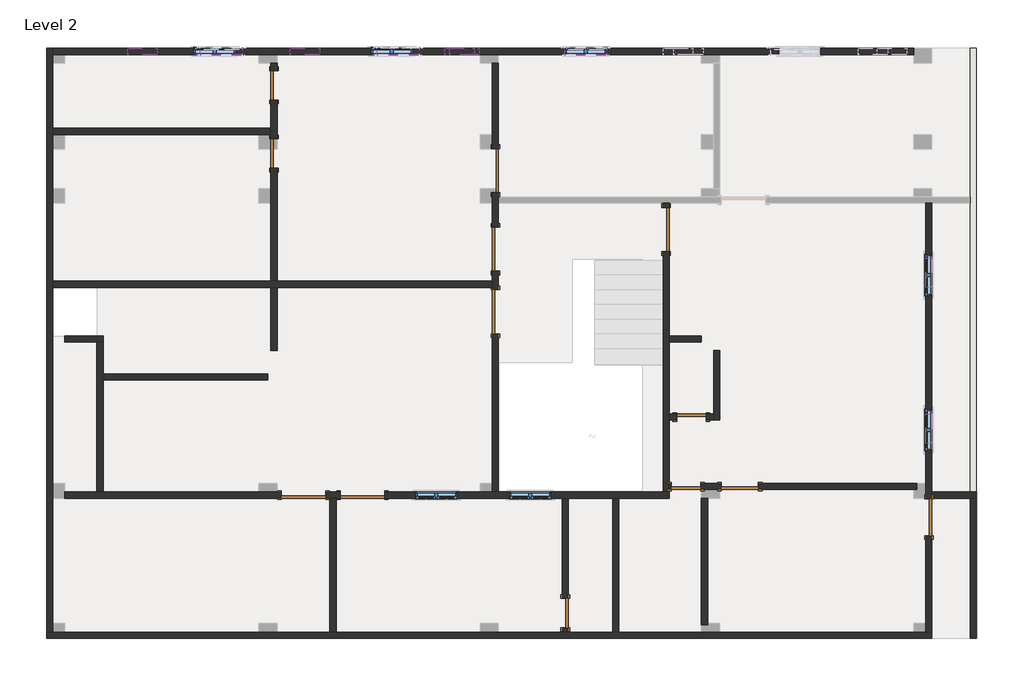
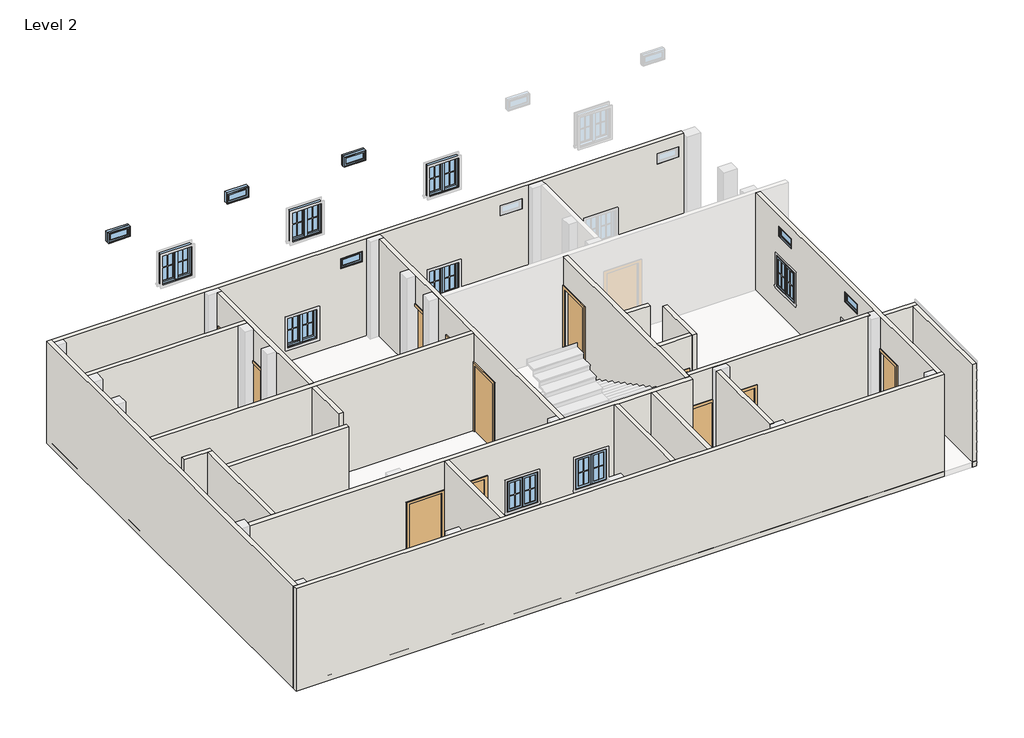
# One storey, part 1 of 2: 24 walls, 16 windows, 13 doors.
"""IFC4 building model written with IfcOpenShell, lengths in millimetres."""

from ifc_helpers import new_model, si_unit, frame, origin, place, context, project, spatial, polyline, outline, extrude, faceted_brep, transform, mapped, element, save
from components import single_flush_2_ccebbf4d, single_flush_2_025d1c86, door_e00f436c, door_1fe7f57d, door_a3eb833a, door_a1797ceb, window_4c2727af, window_0d9958e7

model = new_model("IFC4")

# Units and contexts
model_context = context("Model", 3, world=origin())
ifc_project = project(units=[si_unit("LENGTHUNIT", "METRE", prefix="MILLI")], contexts=[model_context])

# Site, building, storey
site = spatial("IfcSite", under=ifc_project)
building = spatial("IfcBuilding", under=site)
storey = spatial("IfcBuildingStorey", under=building, Name="Level 2", Elevation=3048.0)

# Doors
placement = place(None, origin())
single_flush_2_shape = single_flush_2_ccebbf4d(model_context)
element("IfcDoor", 1, ObjectType="Single-Flush : 2'", at=placement, inside=storey, context=model_context, shape_type="MappedRepresentation", body=[
    mapped(single_flush_2_shape, transform((758.239606, -5823.8831508, 3048.0), x_axis=(1.0, 0.0, 0.0), y_axis=(0.0, 1.0, 0.0), z_axis=(0.0, 0.0, 1.0))),
])
element("IfcDoor", 2, ObjectType="Single-Flush : 2'", at=placement, inside=storey, context=model_context, shape_type="MappedRepresentation", body=[
    mapped(single_flush_2_shape, transform((874.8985263, -4388.7831508, 3048.0), x_axis=(-1.0, 0.0, 0.0), y_axis=(0.0, -1.0, 0.0), z_axis=(0.0, 0.0, 1.0))),
])
single_flush_2_2_shape = single_flush_2_025d1c86(model_context)
element("IfcDoor", 3, ObjectType="Single-Flush : 2'", at=placement, inside=storey, context=model_context, shape_type="MappedRepresentation", body=[
    mapped(single_flush_2_2_shape, transform((-1732.230394, -8440.0831508, 3048.0), x_axis=(0.0, -1.0, 0.0), y_axis=(1.0, 0.0, 0.0), z_axis=(0.0, 0.0, 1.0))),
])
element("IfcDoor", 4, ObjectType="Single-Flush : 2'", at=placement, inside=storey, context=model_context, shape_type="MappedRepresentation", body=[
    mapped(single_flush_2_2_shape, transform((-7746.0425534, 2469.2168492, 3048.0), x_axis=(0.0, 1.0, 0.0), y_axis=(-1.0, 0.0, 0.0), z_axis=(0.0, 0.0, 1.0))),
])
element("IfcDoor", 5, ObjectType="Single-Flush : 2'", at=placement, inside=storey, context=model_context, shape_type="MappedRepresentation", body=[
    mapped(single_flush_2_2_shape, transform((-7746.0425534, 1059.5168492, 3048.0), x_axis=(0.0, 1.0, 0.0), y_axis=(-1.0, 0.0, 0.0), z_axis=(0.0, 0.0, 1.0))),
])
door_shape = door_e00f436c(model_context)
element("IfcDoor", 6, ObjectType="Single-Flush : 30\" x 80\"", at=placement, inside=storey, context=model_context, shape_type="MappedRepresentation", body=[
    mapped(door_shape, transform((5779.4574466, -6458.8831508, 3048.0), x_axis=(0.0, 1.0, 0.0), y_axis=(-1.0, 0.0, 0.0), z_axis=(0.0, 0.0, 1.0))),
])
door_2_shape = door_1fe7f57d(model_context)
element("IfcDoor", 7, ObjectType="Single-Flush : 30\" x 80\"", at=placement, inside=storey, context=model_context, shape_type="MappedRepresentation", body=[
    mapped(door_2_shape, transform((1875.839606, -5823.8831508, 3048.0), x_axis=(-1.0, 0.0, 0.0), y_axis=(0.0, -1.0, 0.0), z_axis=(0.0, 0.0, 1.0))),
])
door_3_shape = door_a3eb833a(model_context)
element("IfcDoor", 8, ObjectType="Single-Flush : 36\" x 84\"", at=placement, inside=storey, context=model_context, shape_type="MappedRepresentation", body=[
    mapped(door_3_shape, transform((-3174.0425534, -919.1431508, 3048.0), x_axis=(0.0, -1.0, 0.0), y_axis=(1.0, 0.0, 0.0), z_axis=(0.0, 0.0, 1.0))),
])
element("IfcDoor", 9, ObjectType="Single-Flush : 36\" x 84\"", at=placement, inside=storey, context=model_context, shape_type="MappedRepresentation", body=[
    mapped(door_3_shape, transform((-7136.4425534, -6001.6831508, 3048.0), x_axis=(1.0, 0.0, 0.0), y_axis=(0.0, 1.0, 0.0), z_axis=(0.0, 0.0, 1.0))),
])
door_4_shape = door_a1797ceb(model_context)
element("IfcDoor", 10, ObjectType="Single-Flush : 36\" x 84\"", at=placement, inside=storey, context=model_context, shape_type="MappedRepresentation", body=[
    mapped(door_4_shape, transform((351.839606, -515.2831508, 3048.0), x_axis=(0.0, -1.0, 0.0), y_axis=(1.0, 0.0, 0.0), z_axis=(0.0, 0.0, 1.0))),
])
element("IfcDoor", 11, ObjectType="Single-Flush : 36\" x 84\"", at=placement, inside=storey, context=model_context, shape_type="MappedRepresentation", body=[
    mapped(door_4_shape, transform((-3174.0425534, 703.9168492, 3048.0), x_axis=(0.0, -1.0, 0.0), y_axis=(1.0, 0.0, 0.0), z_axis=(0.0, 0.0, 1.0))),
])
element("IfcDoor", 12, ObjectType="Single-Flush : 36\" x 84\"", at=placement, inside=storey, context=model_context, shape_type="MappedRepresentation", body=[
    mapped(door_4_shape, transform((-3174.0425534, -2214.5431508, 3048.0), x_axis=(0.0, 1.0, 0.0), y_axis=(-1.0, 0.0, 0.0), z_axis=(0.0, 0.0, 1.0))),
])
element("IfcDoor", 13, ObjectType="Single-Flush : 36\" x 84\"", at=placement, inside=storey, context=model_context, shape_type="MappedRepresentation", body=[
    mapped(door_4_shape, transform((-5917.2425534, -6001.6831508, 3048.0), x_axis=(-1.0, 0.0, 0.0), y_axis=(0.0, -1.0, 0.0), z_axis=(0.0, 0.0, 1.0))),
])

# Walls
element("IfcWall", 14, ObjectType="Generic - 5\"", at=placement, inside=storey, context=model_context, shape_type="Brep", body=[
    faceted_brep([(-12445.0425534, -8960.7831508, 3048.0), (5842.9574466, -8960.7831508, 3048.0), (5842.9574466, -8960.7831508, 6096.0), (-12445.0425534, -8960.7831508, 6096.0), (-12445.0425534, -8833.7831508, 3048.0), (-12445.0425534, -8833.7831508, 6096.0), (-12318.0425534, -8833.7831508, 6096.0), (-6590.3425534, -8833.7831508, 6096.0), (-6463.3425534, -8833.7831508, 6096.0), (-1795.730394, -8833.7831508, 6096.0), (-1668.730394, -8833.7831508, 6096.0), (-754.330394, -8833.7831508, 6096.0), (-627.330394, -8833.7831508, 6096.0), (5715.9574466, -8833.7831508, 6096.0), (5842.9574466, -8833.7831508, 6096.0), (5842.9574466, -8833.7831508, 3048.0), (5715.9574466, -8833.7831508, 3048.0), (-627.330394, -8833.7831508, 3048.0), (-754.330394, -8833.7831508, 3048.0), (-1668.730394, -8833.7831508, 3048.0), (-1795.730394, -8833.7831508, 3048.0), (-6463.3425534, -8833.7831508, 3048.0), (-6590.3425534, -8833.7831508, 3048.0), (-12318.0425534, -8833.7831508, 3048.0)], [[[0, 1, 2, 3]], [[4, 5, 6, 7, 8, 9, 10, 11, 12, 13, 14, 15, 16, 17, 18, 19, 20, 21, 22, 23]], [[1, 0, 4, 23, 22, 21, 20, 19, 18, 17, 16, 15]], [[3, 2, 14, 13, 12, 11, 10, 9, 8, 7, 6, 5]], [[0, 3, 5, 4]], [[2, 1, 15, 14]]]),
])
element("IfcWall", 15, ObjectType="Generic - 5\"", at=placement, inside=storey, context=model_context, shape_type="Brep", body=[
    faceted_brep([(-12318.0425534, -8833.7831508, 3048.0), (-12318.0425534, -1709.0831508, 3048.0), (-12318.0425534, -1582.0831508, 3048.0), (-12318.0425534, 1453.2168492, 3048.0), (-12318.0425534, 1580.2168492, 3048.0), (-12318.0425534, 3104.2168492, 3048.0), (-12318.0425534, 3231.2168492, 3048.0), (-12318.0425534, 3231.2168492, 6096.0), (-12318.0425534, 3104.2168492, 6096.0), (-12318.0425534, 1580.2168492, 6096.0), (-12318.0425534, 1453.2168492, 6096.0), (-12318.0425534, -1582.0831508, 6096.0), (-12318.0425534, -1709.0831508, 6096.0), (-12318.0425534, -8833.7831508, 6096.0), (-12318.0425534, -8833.7831508, 6091.0), (-12318.0425534, -8833.7831508, 3053.0), (-12445.0425534, -8833.7831508, 3048.0), (-12445.0425534, -8833.7831508, 6096.0), (-12445.0425534, 3231.2168492, 6096.0), (-12445.0425534, 3231.2168492, 3048.0)], [[[0, 1, 2, 3, 4, 5, 6, 7, 8, 9, 10, 11, 12, 13, 14, 15]], [[16, 17, 18, 19]], [[6, 5, 4, 3, 2, 1, 0, 16, 19]], [[13, 12, 11, 10, 9, 8, 7, 18, 17]], [[0, 15, 14, 13, 17, 16]], [[7, 6, 19, 18]]]),
])
element("IfcWall", 16, ObjectType="Generic - 5\"", at=placement, inside=storey, context=model_context, shape_type="Brep", body=[
    faceted_brep([(-12318.0425534, 3104.2168492, 3048.0), (5461.9574466, 3104.2168492, 3048.0), (5461.9574466, 3104.2168492, 6096.0), (-12318.0425534, 3104.2168492, 6096.0), (-12318.0425534, 3104.2168492, 6091.0), (-12318.0425534, 3104.2168492, 3053.0), (-4215.4425534, 3104.2168492, 5444.6055795), (-4215.4425534, 3104.2168492, 5749.4055795), (-3605.8425534, 3104.2168492, 5749.4055795), (-3605.8425534, 3104.2168492, 5444.6055795), (288.339606, 3104.2168492, 5444.6055795), (288.339606, 3104.2168492, 5749.4055795), (897.939606, 3104.2168492, 5749.4055795), (897.939606, 3104.2168492, 5444.6055795), (4707.939606, 3104.2168492, 5444.6055795), (4707.939606, 3104.2168492, 5749.4055795), (5317.539606, 3104.2168492, 5749.4055795), (5317.539606, 3104.2168492, 5444.6055795), (-874.980394, 3104.2168492, 4514.85), (-874.980394, 3104.2168492, 3600.45), (-1738.580394, 3104.2168492, 3600.45), (-1738.580394, 3104.2168492, 4514.85), (3544.619606, 3104.2168492, 4514.85), (3544.619606, 3104.2168492, 3600.45), (2681.019606, 3104.2168492, 3600.45), (2681.019606, 3104.2168492, 4514.85), (-4879.0175534, 3104.2168492, 4514.85), (-4879.0175534, 3104.2168492, 3600.45), (-5742.6175534, 3104.2168492, 3600.45), (-5742.6175534, 3104.2168492, 4514.85), (-8536.6175534, 3104.2168492, 4514.85), (-8536.6175534, 3104.2168492, 3600.45), (-9400.2175534, 3104.2168492, 3600.45), (-9400.2175534, 3104.2168492, 4514.85), (5461.9574466, 3231.2168492, 3048.0), (-12318.0425534, 3231.2168492, 3048.0), (-12318.0425534, 3231.2168492, 6096.0), (5461.9574466, 3231.2168492, 6096.0), (5461.9574466, 3231.2168492, 6091.0), (5461.9574466, 3231.2168492, 3053.0), (-4215.4425534, 3231.2168492, 5749.4055795), (-4215.4425534, 3231.2168492, 5444.6055795), (-3605.8425534, 3231.2168492, 5444.6055795), (-3605.8425534, 3231.2168492, 5749.4055795), (288.339606, 3231.2168492, 5749.4055795), (288.339606, 3231.2168492, 5444.6055795), (897.939606, 3231.2168492, 5444.6055795), (897.939606, 3231.2168492, 5749.4055795), (4707.939606, 3231.2168492, 5749.4055795), (4707.939606, 3231.2168492, 5444.6055795), (5317.539606, 3231.2168492, 5444.6055795), (5317.539606, 3231.2168492, 5749.4055795), (-874.980394, 3231.2168492, 3600.45), (-874.980394, 3231.2168492, 4514.85), (-1738.580394, 3231.2168492, 4514.85), (-1738.580394, 3231.2168492, 3600.45), (3544.619606, 3231.2168492, 3600.45), (3544.619606, 3231.2168492, 4514.85), (2681.019606, 3231.2168492, 4514.85), (2681.019606, 3231.2168492, 3600.45), (-4879.0175534, 3231.2168492, 3600.45), (-4879.0175534, 3231.2168492, 4514.85), (-5742.6175534, 3231.2168492, 4514.85), (-5742.6175534, 3231.2168492, 3600.45), (-8536.6175534, 3231.2168492, 3600.45), (-8536.6175534, 3231.2168492, 4514.85), (-9400.2175534, 3231.2168492, 4514.85), (-9400.2175534, 3231.2168492, 3600.45)], [[[0, 1, 2, 3, 4, 5], [6, 7, 8, 9], [10, 11, 12, 13], [14, 15, 16, 17], [18, 19, 20, 21], [22, 23, 24, 25], [26, 27, 28, 29], [30, 31, 32, 33]], [[34, 35, 36, 37, 38, 39], [40, 41, 42, 43], [44, 45, 46, 47], [48, 49, 50, 51], [52, 53, 54, 55], [56, 57, 58, 59], [60, 61, 62, 63], [64, 65, 66, 67]], [[1, 0, 35, 34]], [[2, 1, 34, 39, 38, 37]], [[3, 2, 37, 36]], [[0, 5, 4, 3, 36, 35]], [[40, 7, 6, 41]], [[41, 6, 9, 42]], [[42, 9, 8, 43]], [[7, 40, 43, 8]], [[45, 44, 11, 10]], [[46, 45, 10, 13]], [[47, 46, 13, 12]], [[44, 47, 12, 11]], [[49, 48, 15, 14]], [[50, 49, 14, 17]], [[51, 50, 17, 16]], [[48, 51, 16, 15]], [[18, 53, 52, 19]], [[19, 52, 55, 20]], [[20, 55, 54, 21]], [[53, 18, 21, 54]], [[23, 22, 57, 56]], [[24, 23, 56, 59]], [[25, 24, 59, 58]], [[22, 25, 58, 57]], [[27, 26, 61, 60]], [[28, 27, 60, 63]], [[29, 28, 63, 62]], [[26, 29, 62, 61]], [[31, 30, 65, 64]], [[32, 31, 64, 67]], [[33, 32, 67, 66]], [[30, 33, 66, 65]]]),
])
element("IfcWall", 17, ObjectType="Generic - 5\"", at=placement, inside=storey, context=model_context, shape_type="SweptSolid", body=[
    extrude(outline(polyline([(6630.3574466, -5938.1831508), (6630.3574466, 3231.2168492), (6757.3574466, 3231.2168492), (6757.3574466, -5938.1831508), (6630.3574466, -5938.1831508)])), frame((0.0, 0.0, 3200.4), z_axis=(0.0, 0.0, 1.0), x_axis=(1.0, 0.0, 0.0)), (0.0, 0.0, 1.0), 762.0),
])
element("IfcWall", 18, ObjectType="Generic - 5\"", at=placement, inside=storey, context=model_context, shape_type="Brep", body=[
    faceted_brep([(5715.9574466, -8833.7831508, 6096.0), (5715.9574466, 30.8168492, 6096.0), (5715.9574466, 30.8168492, 3048.0), (5715.9574466, -6077.8831508, 3048.0), (5715.9574466, -6077.8831508, 5080.0), (5715.9574466, -6839.8831508, 5080.0), (5715.9574466, -6839.8831508, 3048.0), (5715.9574466, -8833.7831508, 3048.0), (5715.9574466, -8833.7831508, 3053.0), (5715.9574466, -8833.7831508, 6091.0), (5715.9574466, -4223.6831508, 3962.4), (5715.9574466, -4223.6831508, 4876.8), (5715.9574466, -5087.2831508, 4876.8), (5715.9574466, -5087.2831508, 3962.4), (5715.9574466, -1023.2831508, 3962.4), (5715.9574466, -1023.2831508, 4876.8), (5715.9574466, -1886.8831508, 4876.8), (5715.9574466, -1886.8831508, 3962.4), (5715.9574466, -4325.2831508, 5486.4), (5715.9574466, -4325.2831508, 5791.2), (5715.9574466, -4934.8831508, 5791.2), (5715.9574466, -4934.8831508, 5486.4), (5715.9574466, -1099.4831508, 5486.4), (5715.9574466, -1099.4831508, 5791.2), (5715.9574466, -1709.0831508, 5791.2), (5715.9574466, -1709.0831508, 5486.4), (5842.9574466, 30.8168492, 6096.0), (5842.9574466, -5938.1831508, 6096.0), (5842.9574466, -6065.1831508, 6096.0), (5842.9574466, -8833.7831508, 6096.0), (5842.9574466, -8833.7831508, 3048.0), (5842.9574466, -6839.8831508, 3048.0), (5842.9574466, -6839.8831508, 5080.0), (5842.9574466, -6077.8831508, 5080.0), (5842.9574466, -6077.8831508, 3048.0), (5842.9574466, -6065.1831508, 3048.0), (5842.9574466, -5938.1831508, 3048.0), (5842.9574466, 30.8168492, 3048.0), (5842.9574466, -4223.6831508, 4876.8), (5842.9574466, -4223.6831508, 3962.4), (5842.9574466, -5087.2831508, 3962.4), (5842.9574466, -5087.2831508, 4876.8), (5842.9574466, -1023.2831508, 4876.8), (5842.9574466, -1023.2831508, 3962.4), (5842.9574466, -1886.8831508, 3962.4), (5842.9574466, -1886.8831508, 4876.8), (5842.9574466, -4325.2831508, 5791.2), (5842.9574466, -4325.2831508, 5486.4), (5842.9574466, -4934.8831508, 5486.4), (5842.9574466, -4934.8831508, 5791.2), (5842.9574466, -1099.4831508, 5791.2), (5842.9574466, -1099.4831508, 5486.4), (5842.9574466, -1709.0831508, 5486.4), (5842.9574466, -1709.0831508, 5791.2)], [[[0, 1, 2, 3, 4, 5, 6, 7, 8, 9], [10, 11, 12, 13], [14, 15, 16, 17], [18, 19, 20, 21], [22, 23, 24, 25]], [[26, 27, 28, 29, 30, 31, 32, 33, 34, 35, 36, 37], [38, 39, 40, 41], [42, 43, 44, 45], [46, 47, 48, 49], [50, 51, 52, 53]], [[30, 7, 6, 31]], [[2, 37, 36, 35, 34, 3]], [[1, 0, 29, 28, 27, 26]], [[0, 9, 8, 7, 30, 29]], [[2, 1, 26, 37]], [[4, 3, 34, 33]], [[5, 4, 33, 32]], [[6, 5, 32, 31]], [[39, 38, 11, 10]], [[40, 39, 10, 13]], [[41, 40, 13, 12]], [[38, 41, 12, 11]], [[43, 42, 15, 14]], [[44, 43, 14, 17]], [[45, 44, 17, 16]], [[42, 45, 16, 15]], [[46, 19, 18, 47]], [[47, 18, 21, 48]], [[48, 21, 20, 49]], [[19, 46, 49, 20]], [[51, 50, 23, 22]], [[52, 51, 22, 25]], [[53, 52, 25, 24]], [[50, 53, 24, 23]]]),
])
element("IfcWall", 19, ObjectType="Generic - 5\"", at=placement, inside=storey, context=model_context, shape_type="Brep", body=[
    faceted_brep([(415.339606, -5938.1831508, 3048.0), (415.339606, -5887.3831508, 3048.0), (415.339606, -5760.3831508, 3048.0), (415.339606, -4452.2831508, 3048.0), (415.339606, -4325.2831508, 3048.0), (415.339606, -2839.3831508, 3048.0), (415.339606, -2712.3831508, 3048.0), (415.339606, -972.4831508, 3048.0), (415.339606, -972.4831508, 5181.6), (415.339606, -58.0831508, 5181.6), (415.339606, -58.0831508, 3048.0), (415.339606, 30.8168492, 3048.0), (415.339606, 30.8168492, 6096.0), (415.339606, -2712.3831508, 6096.0), (415.339606, -2839.3831508, 6096.0), (415.339606, -4325.2831508, 6096.0), (415.339606, -4452.2831508, 6096.0), (415.339606, -5760.3831508, 6096.0), (415.339606, -5887.3831508, 6096.0), (415.339606, -5938.1831508, 6096.0), (288.339606, -972.4831508, 5181.6), (288.339606, -972.4831508, 3048.0), (288.339606, -5938.1831508, 3048.0), (288.339606, -5938.1831508, 6096.0), (288.339606, 30.8168492, 6096.0), (288.339606, 30.8168492, 3048.0), (288.339606, -58.0831508, 3048.0), (288.339606, -58.0831508, 5181.6)], [[[0, 1, 2, 3, 4, 5, 6, 7, 8, 9, 10, 11, 12, 13, 14, 15, 16, 17, 18, 19]], [[20, 21, 22, 23, 24, 25, 26, 27]], [[26, 25, 11, 10]], [[22, 21, 7, 6, 5, 4, 3, 2, 1, 0]], [[19, 18, 17, 16, 15, 14, 13, 12, 24, 23]], [[0, 19, 23, 22]], [[12, 11, 25, 24]], [[8, 7, 21, 20]], [[9, 8, 20, 27]], [[10, 9, 27, 26]]]),
])
element("IfcWall", 20, ObjectType="Generic - 5\"", at=placement, inside=storey, context=model_context, shape_type="SweptSolid", body=[
    extrude(outline(polyline([(415.339606, -2712.3831508), (1080.4574466, -2712.3831508), (1080.4574466, -2839.3831508), (415.339606, -2839.3831508), (415.339606, -2712.3831508)])), frame((0.0, 0.0, 3048.0), z_axis=(0.0, 0.0, 1.0), x_axis=(1.0, 0.0, 0.0)), (0.0, 0.0, 1.0), 3048.0),
])
element("IfcWall", 21, ObjectType="Generic - 5\"", at=placement, inside=storey, context=model_context, shape_type="Brep", body=[
    faceted_brep([(-3237.5425534, -1376.3431508, 5181.6), (-3237.5425534, -1376.3431508, 3048.0), (-3237.5425534, -1582.0831508, 3048.0), (-3237.5425534, -1709.0831508, 3048.0), (-3237.5425534, -1757.3431508, 3048.0), (-3237.5425534, -1757.3431508, 5181.6), (-3237.5425534, -2671.7431508, 5181.6), (-3237.5425534, -2671.7431508, 3048.0), (-3237.5425534, -5938.1831508, 3048.0), (-3237.5425534, -5938.1831508, 3053.0), (-3237.5425534, -5938.1831508, 6091.0), (-3237.5425534, -5938.1831508, 6096.0), (-3237.5425534, -1709.0831508, 6096.0), (-3237.5425534, -1582.0831508, 6096.0), (-3237.5425534, 2926.4168492, 6096.0), (-3237.5425534, 2926.4168492, 3048.0), (-3237.5425534, 1161.1168492, 3048.0), (-3237.5425534, 1161.1168492, 3053.0), (-3237.5425534, 1161.1168492, 5181.6), (-3237.5425534, 1144.8754758, 5181.6), (-3237.5425534, 335.6168492, 5181.6), (-3237.5425534, 246.7168492, 5181.6), (-3237.5425534, 246.7168492, 3053.0), (-3237.5425534, 246.7168492, 3048.0), (-3237.5425534, -461.9431508, 3048.0), (-3237.5425534, -461.9431508, 5181.6), (-3110.5425534, -1757.3431508, 3048.0), (-3110.5425534, -1376.3431508, 3048.0), (-3110.5425534, -1376.3431508, 5181.6), (-3110.5425534, -461.9431508, 5181.6), (-3110.5425534, -461.9431508, 3048.0), (-3110.5425534, 30.8168492, 3048.0), (-3110.5425534, 157.8168492, 3048.0), (-3110.5425534, 246.7168492, 3048.0), (-3110.5425534, 246.7168492, 3053.0), (-3110.5425534, 246.7168492, 5181.6), (-3110.5425534, 335.6168492, 5181.6), (-3110.5425534, 1144.8754758, 5181.6), (-3110.5425534, 1161.1168492, 5181.6), (-3110.5425534, 1161.1168492, 3053.0), (-3110.5425534, 1161.1168492, 3048.0), (-3110.5425534, 2926.4168492, 3048.0), (-3110.5425534, 2926.4168492, 3053.0), (-3110.5425534, 2926.4168492, 6091.0), (-3110.5425534, 2926.4168492, 6096.0), (-3110.5425534, 157.8168492, 6096.0), (-3110.5425534, 30.8168492, 6096.0), (-3110.5425534, -5938.1831508, 6096.0), (-3110.5425534, -5938.1831508, 3048.0), (-3110.5425534, -2671.7431508, 3048.0), (-3110.5425534, -2671.7431508, 5181.6), (-3110.5425534, -1757.3431508, 5181.6)], [[[0, 1, 2, 3, 4, 5, 6, 7, 8, 9, 10, 11, 12, 13, 14, 15, 16, 17, 18, 19, 20, 21, 22, 23, 24, 25]], [[26, 27, 28, 29, 30, 31, 32, 33, 34, 35, 36, 37, 38, 39, 40, 41, 42, 43, 44, 45, 46, 47, 48, 49, 50, 51]], [[16, 15, 41, 40]], [[49, 48, 8, 7]], [[24, 23, 33, 32, 31, 30]], [[4, 3, 2, 1, 27, 26]], [[14, 13, 12, 11, 47, 46, 45, 44]], [[15, 14, 44, 43, 42, 41]], [[35, 34, 33, 23, 22, 21]], [[38, 37, 36, 35, 21, 20, 19, 18]], [[40, 39, 38, 18, 17, 16]], [[11, 10, 9, 8, 48, 47]], [[5, 4, 26, 51]], [[6, 5, 51, 50]], [[7, 6, 50, 49]], [[28, 27, 1, 0]], [[29, 28, 0, 25]], [[30, 29, 25, 24]]]),
])
element("IfcWall", 22, ObjectType="Generic - 5\"", at=placement, inside=storey, context=model_context, shape_type="Brep", body=[
    faceted_brep([(-3237.5425534, -1582.0831508, 3048.0), (-7682.5425534, -1582.0831508, 3048.0), (-7809.5425534, -1582.0831508, 3048.0), (-12318.0425534, -1582.0831508, 3048.0), (-12318.0425534, -1582.0831508, 6096.0), (-7809.5425534, -1582.0831508, 6096.0), (-7682.5425534, -1582.0831508, 6096.0), (-3237.5425534, -1582.0831508, 6096.0), (-3237.5425534, -1709.0831508, 3048.0), (-3237.5425534, -1709.0831508, 6096.0), (-7682.5425534, -1709.0831508, 6096.0), (-7809.5425534, -1709.0831508, 6096.0), (-12318.0425534, -1709.0831508, 6096.0), (-12318.0425534, -1709.0831508, 3048.0), (-7809.5425534, -1709.0831508, 3048.0), (-7682.5425534, -1709.0831508, 3048.0), (-3237.5425534, -1655.7431508, 3048.0)], [[[0, 1, 2, 3, 4, 5, 6, 7]], [[8, 9, 10, 11, 12, 13, 14, 15]], [[3, 2, 1, 0, 16, 8, 15, 14, 13]], [[7, 6, 5, 4, 12, 11, 10, 9]], [[0, 7, 9, 8, 16]], [[4, 3, 13, 12]]]),
])
element("IfcWall", 23, ObjectType="Generic - 5\"", at=placement, inside=storey, context=model_context, shape_type="SweptSolid", body=[
    extrude(outline(polyline([(-754.330394, -8833.7831508), (-754.330394, -6065.1831508), (-627.330394, -6065.1831508), (-627.330394, -8833.7831508), (-754.330394, -8833.7831508)])), frame((0.0, 0.0, 3048.0), z_axis=(0.0, 0.0, 1.0), x_axis=(1.0, 0.0, 0.0)), (0.0, 0.0, 1.0), 3048.0),
])
element("IfcWall", 24, ObjectType="Generic - 5\"", at=placement, inside=storey, context=model_context, shape_type="Brep", body=[
    faceted_brep([(-6679.2425534, -6065.1831508, 3048.0), (-6590.3425534, -6065.1831508, 3048.0), (-6463.3425534, -6065.1831508, 3048.0), (-6374.4425534, -6065.1831508, 3048.0), (-6374.4425534, -6065.1831508, 5181.6), (-5460.0425534, -6065.1831508, 5181.6), (-5460.0425534, -6065.1831508, 3048.0), (-1795.730394, -6065.1831508, 3048.0), (-1668.730394, -6065.1831508, 3048.0), (-754.330394, -6065.1831508, 3048.0), (-627.330394, -6065.1831508, 3048.0), (415.339606, -6065.1831508, 3048.0), (415.339606, -6065.1831508, 6096.0), (-627.330394, -6065.1831508, 6096.0), (-754.330394, -6065.1831508, 6096.0), (-1668.730394, -6065.1831508, 6096.0), (-1795.730394, -6065.1831508, 6096.0), (-6463.3425534, -6065.1831508, 6096.0), (-6590.3425534, -6065.1831508, 6096.0), (-12064.0425534, -6065.1831508, 6096.0), (-12064.0425534, -6065.1831508, 6091.0), (-12064.0425534, -6065.1831508, 3053.0), (-12064.0425534, -6065.1831508, 3048.0), (-7593.6425534, -6065.1831508, 3048.0), (-7593.6425534, -6065.1831508, 5181.6), (-6679.2425534, -6065.1831508, 5181.6), (-4825.0425534, -6065.1831508, 4876.8), (-3961.4425534, -6065.1831508, 4876.8), (-3961.4425534, -6065.1831508, 3962.4), (-4825.0425534, -6065.1831508, 3962.4), (-2884.9364737, -6065.1831508, 4876.8), (-2021.3364737, -6065.1831508, 4876.8), (-2021.3364737, -6065.1831508, 3962.4), (-2884.9364737, -6065.1831508, 3962.4), (-6374.4425534, -5938.1831508, 5181.6), (-6374.4425534, -5938.1831508, 3048.0), (-6679.2425534, -5938.1831508, 3048.0), (-6679.2425534, -5938.1831508, 5181.6), (-7593.6425534, -5938.1831508, 5181.6), (-7593.6425534, -5938.1831508, 3048.0), (-12064.0425534, -5938.1831508, 3048.0), (-12064.0425534, -5938.1831508, 6096.0), (-3237.5425534, -5938.1831508, 6096.0), (-3110.5425534, -5938.1831508, 6096.0), (288.339606, -5938.1831508, 6096.0), (415.339606, -5938.1831508, 6096.0), (415.339606, -5938.1831508, 3048.0), (288.339606, -5938.1831508, 3048.0), (-3110.5425534, -5938.1831508, 3048.0), (-3237.5425534, -5938.1831508, 3048.0), (-5460.0425534, -5938.1831508, 3048.0), (-5460.0425534, -5938.1831508, 5181.6), (-4825.0425534, -5938.1831508, 4876.8), (-4825.0425534, -5938.1831508, 3962.4), (-3961.4425534, -5938.1831508, 3962.4), (-3961.4425534, -5938.1831508, 4876.8), (-2884.9364737, -5938.1831508, 4876.8), (-2884.9364737, -5938.1831508, 3962.4), (-2021.3364737, -5938.1831508, 3962.4), (-2021.3364737, -5938.1831508, 4876.8)], [[[0, 1, 2, 3, 4, 5, 6, 7, 8, 9, 10, 11, 12, 13, 14, 15, 16, 17, 18, 19, 20, 21, 22, 23, 24, 25], [26, 27, 28, 29], [30, 31, 32, 33]], [[34, 35, 36, 37, 38, 39, 40, 41, 42, 43, 44, 45, 46, 47, 48, 49, 50, 51], [52, 53, 54, 55], [56, 57, 58, 59]], [[23, 22, 40, 39]], [[36, 35, 3, 2, 1, 0]], [[50, 49, 48, 47, 46, 11, 10, 9, 8, 7, 6]], [[19, 18, 17, 16, 15, 14, 13, 12, 45, 44, 43, 42, 41]], [[22, 21, 20, 19, 41, 40]], [[12, 11, 46, 45]], [[37, 36, 0, 25]], [[38, 37, 25, 24]], [[39, 38, 24, 23]], [[4, 3, 35, 34]], [[5, 4, 34, 51]], [[6, 5, 51, 50]], [[53, 52, 26, 29]], [[54, 53, 29, 28]], [[55, 54, 28, 27]], [[52, 55, 27, 26]], [[57, 56, 30, 33]], [[58, 57, 33, 32]], [[59, 58, 32, 31]], [[56, 59, 31, 30]]]),
])
element("IfcWall", 25, ObjectType="Generic - 5\"", at=placement, inside=storey, context=model_context, shape_type="Brep", body=[
    faceted_brep([(1080.4574466, -6065.1831508, 3048.0), (1080.4574466, -8681.3831508, 3048.0), (1080.4574466, -8681.3831508, 3053.0), (1080.4574466, -8681.3831508, 6091.0), (1080.4574466, -8681.3831508, 6096.0), (1080.4574466, -6065.1831508, 6096.0), (1080.4574466, -6065.1831508, 6091.0), (1080.4574466, -6065.1831508, 3053.0), (1207.4574466, -6065.1831508, 3048.0), (1207.4574466, -6065.1831508, 6096.0), (1207.4574466, -8681.3831508, 6096.0), (1207.4574466, -8681.3831508, 6091.0), (1207.4574466, -8681.3831508, 3053.0), (1207.4574466, -8681.3831508, 3048.0)], [[[0, 1, 2, 3, 4, 5, 6, 7]], [[8, 9, 10, 11, 12, 13]], [[1, 0, 8, 13]], [[4, 3, 2, 1, 13, 12, 11, 10]], [[5, 4, 10, 9]], [[0, 7, 6, 5, 9, 8]]]),
])
element("IfcWall", 26, ObjectType="Generic - 5\"", at=placement, inside=storey, context=model_context, shape_type="Brep", body=[
    faceted_brep([(1494.839606, -5760.3831508, 3048.0), (1063.039606, -5760.3831508, 3048.0), (1063.039606, -5760.3831508, 5080.0), (453.439606, -5760.3831508, 5080.0), (453.439606, -5760.3831508, 3048.0), (415.339606, -5760.3831508, 3048.0), (415.339606, -5760.3831508, 6096.0), (5533.439606, -5760.3831508, 6096.0), (5533.439606, -5760.3831508, 6091.0), (5533.439606, -5760.3831508, 3053.0), (5533.439606, -5760.3831508, 3048.0), (2256.839606, -5760.3831508, 3048.0), (2256.839606, -5760.3831508, 5080.0), (1494.839606, -5760.3831508, 5080.0), (1063.039606, -5887.3831508, 5080.0), (1063.039606, -5887.3831508, 3048.0), (1494.839606, -5887.3831508, 3048.0), (1494.839606, -5887.3831508, 5080.0), (2256.839606, -5887.3831508, 5080.0), (2256.839606, -5887.3831508, 3048.0), (5533.439606, -5887.3831508, 3048.0), (5533.439606, -5887.3831508, 3053.0), (5533.439606, -5887.3831508, 6091.0), (5533.439606, -5887.3831508, 6096.0), (415.339606, -5887.3831508, 6096.0), (415.339606, -5887.3831508, 3048.0), (453.439606, -5887.3831508, 3048.0), (453.439606, -5887.3831508, 5080.0)], [[[0, 1, 2, 3, 4, 5, 6, 7, 8, 9, 10, 11, 12, 13]], [[14, 15, 16, 17, 18, 19, 20, 21, 22, 23, 24, 25, 26, 27]], [[11, 10, 20, 19]], [[26, 25, 5, 4]], [[16, 15, 1, 0]], [[7, 6, 24, 23]], [[10, 9, 8, 7, 23, 22, 21, 20]], [[6, 5, 25, 24]], [[17, 16, 0, 13]], [[18, 17, 13, 12]], [[19, 18, 12, 11]], [[2, 1, 15, 14]], [[3, 2, 14, 27]], [[4, 3, 27, 26]]]),
])
element("IfcWall", 27, ObjectType="Generic - 5\"", at=placement, inside=storey, context=model_context, shape_type="Brep", body=[
    faceted_brep([(1334.4574466, -3017.1831508, 3048.0), (1334.4574466, -4325.2831508, 3048.0), (1334.4574466, -4452.2831508, 3048.0), (1334.4574466, -4452.2831508, 6096.0), (1334.4574466, -4325.2831508, 6096.0), (1334.4574466, -3017.1831508, 6096.0), (1461.4574466, -3017.1831508, 3048.0), (1461.4574466, -3017.1831508, 6096.0), (1461.4574466, -4452.2831508, 6096.0), (1461.4574466, -4452.2831508, 3048.0)], [[[0, 1, 2, 3, 4, 5]], [[6, 7, 8, 9]], [[2, 1, 0, 6, 9]], [[5, 4, 3, 8, 7]], [[0, 5, 7, 6]], [[3, 2, 9, 8]]]),
])
element("IfcWall", 28, ObjectType="Generic - 5\"", at=placement, inside=storey, context=model_context, shape_type="SweptSolid", body=[
    extrude(outline(polyline([(3048.0, 415.339606), (3048.0, 570.0985263), (5080.0, 570.0985263), (5080.0, 1179.6985263), (3048.0, 1179.6985263), (3048.0, 1334.4574466), (6096.0, 1334.4574466), (6096.0, 415.339606), (3048.0, 415.339606)])), frame((0.0, -4452.2831508, 0.0), z_axis=(0.0, 1.0, 0.0), x_axis=(0.0, 0.0, 1.0)), (0.0, 0.0, 1.0), 127.0),
])
element("IfcWall", 29, ObjectType="Generic - 5\"", at=placement, inside=storey, context=model_context, shape_type="Brep", body=[
    faceted_brep([(5842.9574466, -6065.1831508, 3048.0), (6630.3574466, -6065.1831508, 3048.0), (6757.3574466, -6065.1831508, 3048.0), (6757.3574466, -6065.1831508, 6096.0), (6630.3574466, -6065.1831508, 6096.0), (5842.9574466, -6065.1831508, 6096.0), (5842.9574466, -5938.1831508, 3048.0), (5842.9574466, -5938.1831508, 6096.0), (6757.3574466, -5938.1831508, 6096.0), (6757.3574466, -5938.1831508, 3962.4), (6757.3574466, -5938.1831508, 3200.4), (6757.3574466, -5938.1831508, 3048.0)], [[[0, 1, 2, 3, 4, 5]], [[6, 7, 8, 9, 10, 11]], [[2, 1, 0, 6, 11]], [[5, 4, 3, 8, 7]], [[0, 5, 7, 6]], [[2, 11, 10, 9, 8, 3]]]),
])
element("IfcWall", 30, ObjectType="Generic - 5\"", at=placement, inside=storey, context=model_context, shape_type="SweptSolid", body=[
    extrude(outline(polyline([(6630.3574466, -8960.7831508), (6630.3574466, -6065.1831508), (6757.3574466, -6065.1831508), (6757.3574466, -8960.7831508), (6630.3574466, -8960.7831508)])), frame((0.0, 0.0, 3048.0), z_axis=(0.0, 0.0, 1.0), x_axis=(1.0, 0.0, 0.0)), (0.0, 0.0, 1.0), 3048.0),
])
element("IfcWall", 31, ObjectType="Generic - 5\"", at=placement, inside=storey, context=model_context, shape_type="Brep", body=[
    faceted_brep([(-7809.5425534, -3017.1831508, 3048.0), (-7809.5425534, -3017.1831508, 6096.0), (-7809.5425534, -1709.0831508, 6096.0), (-7809.5425534, -1709.0831508, 3048.0), (-7682.5425534, -3017.1831508, 6096.0), (-7682.5425534, -3017.1831508, 3048.0), (-7682.5425534, -1709.0831508, 3048.0), (-7682.5425534, -1709.0831508, 6096.0)], [[[0, 1, 2, 3]], [[4, 5, 6, 7]], [[5, 0, 3, 6]], [[1, 0, 5, 4]], [[1, 4, 7, 2]], [[3, 2, 7, 6]]]),
    faceted_brep([(-7809.5425534, 2926.4168492, 6096.0), (-7809.5425534, 2926.4168492, 3048.0), (-7809.5425534, 2774.0168492, 3048.0), (-7809.5425534, 2774.0168492, 5080.0), (-7809.5425534, 2164.4168492, 5080.0), (-7809.5425534, 2164.4168492, 3048.0), (-7809.5425534, 1580.2168492, 3048.0), (-7809.5425534, 1453.2168492, 3048.0), (-7809.5425534, 1364.3168492, 3048.0), (-7809.5425534, 1364.3168492, 3053.0), (-7809.5425534, 1364.3168492, 5080.0), (-7809.5425534, 1144.8754758, 5080.0), (-7809.5425534, 754.7168492, 5080.0), (-7809.5425534, 754.7168492, 3048.0), (-7809.5425534, -1582.0831508, 3048.0), (-7809.5425534, -1582.0831508, 6096.0), (-7809.5425534, 1453.2168492, 6096.0), (-7809.5425534, 1580.2168492, 6096.0), (-7682.5425534, 2926.4168492, 3048.0), (-7682.5425534, 2926.4168492, 3053.0), (-7682.5425534, 2926.4168492, 6091.0), (-7682.5425534, 2926.4168492, 6096.0), (-7682.5425534, -1582.0831508, 6096.0), (-7682.5425534, -1582.0831508, 3048.0), (-7682.5425534, 754.7168492, 3048.0), (-7682.5425534, 754.7168492, 5080.0), (-7682.5425534, 1144.8754758, 5080.0), (-7682.5425534, 1364.3168492, 5080.0), (-7682.5425534, 1364.3168492, 3053.0), (-7682.5425534, 1364.3168492, 3048.0), (-7682.5425534, 2164.4168492, 3048.0), (-7682.5425534, 2164.4168492, 5080.0), (-7682.5425534, 2774.0168492, 5080.0), (-7682.5425534, 2774.0168492, 3048.0)], [[[0, 1, 2, 3, 4, 5, 6, 7, 8, 9, 10, 11, 12, 13, 14, 15, 16, 17]], [[18, 19, 20, 21, 22, 23, 24, 25, 26, 27, 28, 29, 30, 31, 32, 33]], [[1, 18, 33, 2]], [[5, 30, 29, 8, 7, 6]], [[13, 24, 23, 14]], [[21, 0, 17, 16, 15, 22]], [[1, 0, 21, 20, 19, 18]], [[15, 14, 23, 22]], [[3, 2, 33, 32]], [[4, 3, 32, 31]], [[5, 4, 31, 30]], [[10, 9, 8, 29, 28, 27]], [[12, 11, 10, 27, 26, 25]], [[13, 12, 25, 24]]]),
])
element("IfcWall", 32, ObjectType="Generic - 5\"", at=placement, inside=storey, context=model_context, shape_type="SweptSolid", body=[
    extrude(outline(polyline([(-6590.3425534, -8833.7831508), (-6590.3425534, -6065.1831508), (-6463.3425534, -6065.1831508), (-6463.3425534, -8833.7831508), (-6590.3425534, -8833.7831508)])), frame((0.0, 0.0, 3048.0), z_axis=(0.0, 0.0, 1.0), x_axis=(1.0, 0.0, 0.0)), (0.0, 0.0, 1.0), 3048.0),
])
element("IfcWall", 33, ObjectType="Generic - 5\"", at=placement, inside=storey, context=model_context, shape_type="SweptSolid", body=[
    extrude(outline(polyline([(-8744.8831508, 5080.0), (-8744.8831508, 3048.0), (-8833.7831508, 3048.0), (-8833.7831508, 6096.0), (-6065.1831508, 6096.0), (-6065.1831508, 3048.0), (-8135.2831508, 3048.0), (-8135.2831508, 5080.0), (-8744.8831508, 5080.0)])), frame((-1795.730394, 0.0, 0.0), z_axis=(1.0, 0.0, 0.0), x_axis=(0.0, 1.0, 0.0)), (0.0, 0.0, 1.0), 127.0),
])
element("IfcWall", 34, ObjectType="Generic - 5\"", at=placement, inside=storey, context=model_context, shape_type="SweptSolid", body=[
    extrude(outline(polyline([(-12318.0425534, 1580.2168492), (-7809.5425534, 1580.2168492), (-7809.5425534, 1453.2168492), (-12318.0425534, 1453.2168492), (-12318.0425534, 1580.2168492)])), frame((0.0, 0.0, 3048.0), z_axis=(0.0, 0.0, 1.0), x_axis=(1.0, 0.0, 0.0)), (0.0, 0.0, 1.0), 3048.0),
])
element("IfcWall", 35, ObjectType="Generic - 5\"", at=placement, inside=storey, context=model_context, shape_type="SweptSolid", body=[
    extrude(outline(polyline([(-11276.6425534, -3499.7831508), (-7873.0425534, -3499.7831508), (-7873.0425534, -3626.7831508), (-11276.6425534, -3626.7831508), (-11276.6425534, -3499.7831508)])), frame((0.0, 0.0, 3048.0), z_axis=(0.0, 0.0, 1.0), x_axis=(1.0, 0.0, 0.0)), (0.0, 0.0, 1.0), 3048.0),
])
element("IfcWall", 36, ObjectType="Generic - 5\"", at=placement, inside=storey, context=model_context, shape_type="Brep", body=[
    faceted_brep([(-12064.0425534, -2839.3831508, 3048.0), (-11403.6425534, -2839.3831508, 3048.0), (-11276.6425534, -2839.3831508, 3048.0), (-11276.6425534, -2839.3831508, 6096.0), (-11403.6425534, -2839.3831508, 6096.0), (-12064.0425534, -2839.3831508, 6096.0), (-12064.0425534, -2712.3831508, 3048.0), (-12064.0425534, -2712.3831508, 6096.0), (-11276.6425534, -2712.3831508, 6096.0), (-11276.6425534, -2712.3831508, 3048.0)], [[[0, 1, 2, 3, 4, 5]], [[6, 7, 8, 9]], [[2, 1, 0, 6, 9]], [[5, 4, 3, 8, 7]], [[0, 5, 7, 6]], [[3, 2, 9, 8]]]),
])
element("IfcWall", 37, ObjectType="Generic - 5\"", at=placement, inside=storey, context=model_context, shape_type="Brep", body=[
    faceted_brep([(-11403.6425534, -2839.3831508, 3048.0), (-11403.6425534, -5912.7831508, 3048.0), (-11403.6425534, -5912.7831508, 6096.0), (-11403.6425534, -2839.3831508, 6096.0), (-11276.6425534, -2839.3831508, 3048.0), (-11276.6425534, -2839.3831508, 6096.0), (-11276.6425534, -3499.7831508, 6096.0), (-11276.6425534, -3626.7831508, 6096.0), (-11276.6425534, -5912.7831508, 6096.0), (-11276.6425534, -5912.7831508, 3048.0), (-11276.6425534, -3626.7831508, 3048.0), (-11276.6425534, -3499.7831508, 3048.0)], [[[0, 1, 2, 3]], [[4, 5, 6, 7, 8, 9, 10, 11]], [[1, 0, 4, 11, 10, 9]], [[2, 1, 9, 8]], [[3, 2, 8, 7, 6, 5]], [[0, 3, 5, 4]]]),
])

# Windows
window_shape = window_4c2727af(model_context)
element("IfcWindow", 38, ObjectType="Fixed : 24\" x 12\"", at=placement, inside=storey, context=model_context, shape_type="MappedRepresentation", body=[
    mapped(window_shape, transform((5779.4574466, -4591.9831508, 4572.0), x_axis=(0.0, 1.0, 0.0), y_axis=(-1.0, 0.0, 0.0), z_axis=(0.0, 0.0, 1.0))),
])
element("IfcWindow", 39, ObjectType="Fixed : 24\" x 12\"", at=placement, inside=storey, context=model_context, shape_type="MappedRepresentation", body=[
    mapped(window_shape, transform((5779.4574466, -1366.1831508, 4572.0), x_axis=(0.0, 1.0, 0.0), y_axis=(-1.0, 0.0, 0.0), z_axis=(0.0, 0.0, 1.0))),
])
element("IfcWindow", 40, ObjectType="Fixed : 24\" x 12\"", at=placement, inside=storey, context=model_context, shape_type="MappedRepresentation", body=[
    mapped(window_shape, transform((-3853.4925534, 3167.7168492, 7521.0555795), x_axis=(-1.0, 0.0, 0.0), y_axis=(0.0, -1.0, 0.0), z_axis=(0.0, 0.0, 1.0))),
])
element("IfcWindow", 41, ObjectType="Fixed : 24\" x 12\"", at=placement, inside=storey, context=model_context, shape_type="MappedRepresentation", body=[
    mapped(window_shape, transform((-3948.7425534, 3167.7168492, 4530.2055795), x_axis=(-1.0, 0.0, 0.0), y_axis=(0.0, -1.0, 0.0), z_axis=(0.0, 0.0, 1.0))),
])
element("IfcWindow", 42, ObjectType="Fixed : 24\" x 12\"", at=placement, inside=storey, context=model_context, shape_type="MappedRepresentation", body=[
    mapped(window_shape, transform((-7149.1425534, 3167.7168492, 7578.2055795), x_axis=(-1.0, 0.0, 0.0), y_axis=(0.0, -1.0, 0.0), z_axis=(0.0, 0.0, 1.0))),
])
element("IfcWindow", 43, ObjectType="Fixed : 24\" x 12\"", at=placement, inside=storey, context=model_context, shape_type="MappedRepresentation", body=[
    mapped(window_shape, transform((-10501.9425534, 3167.7168492, 7578.2055795), x_axis=(-1.0, 0.0, 0.0), y_axis=(0.0, -1.0, 0.0), z_axis=(0.0, 0.0, 1.0))),
])
window_2_shape = window_0d9958e7(model_context)
element("IfcWindow", 44, ObjectType="Window-Casement-Double : 34\" x 36\"", at=placement, inside=storey, context=model_context, shape_type="MappedRepresentation", body=[
    mapped(window_2_shape, transform((-4393.2425534, -6001.6831508, 3048.0), x_axis=(-1.0, 0.0, 0.0), y_axis=(0.0, -1.0, 0.0), z_axis=(0.0, 0.0, 1.0))),
])
element("IfcWindow", 45, ObjectType="Window-Casement-Double : 34\" x 36\"", at=placement, inside=storey, context=model_context, shape_type="MappedRepresentation", body=[
    mapped(window_2_shape, transform((-2453.1364737, -6001.6831508, 3048.0), x_axis=(-1.0, 0.0, 0.0), y_axis=(0.0, -1.0, 0.0), z_axis=(0.0, 0.0, 1.0))),
])
element("IfcWindow", 46, ObjectType="Window-Casement-Double : 34\" x 36\"", at=placement, inside=storey, context=model_context, shape_type="MappedRepresentation", body=[
    mapped(window_2_shape, transform((5779.4574466, -4655.4831508, 3048.0), x_axis=(0.0, 1.0, 0.0), y_axis=(-1.0, 0.0, 0.0), z_axis=(0.0, 0.0, 1.0))),
])
element("IfcWindow", 47, ObjectType="Window-Casement-Double : 34\" x 36\"", at=placement, inside=storey, context=model_context, shape_type="MappedRepresentation", body=[
    mapped(window_2_shape, transform((5779.4574466, -1455.0831508, 3048.0), x_axis=(0.0, 1.0, 0.0), y_axis=(-1.0, 0.0, 0.0), z_axis=(0.0, 0.0, 1.0))),
])
element("IfcWindow", 48, ObjectType="Window-Casement-Double : 34\" x 36\"", at=placement, inside=storey, context=model_context, shape_type="MappedRepresentation", body=[
    mapped(window_2_shape, transform((-1306.780394, 3167.7168492, 5790.1023039), x_axis=(1.0, 0.0, 0.0), y_axis=(0.0, 1.0, 0.0), z_axis=(0.0, 0.0, 1.0))),
])
element("IfcWindow", 49, ObjectType="Window-Casement-Double : 34\" x 36\"", at=placement, inside=storey, context=model_context, shape_type="MappedRepresentation", body=[
    mapped(window_2_shape, transform((-1306.780394, 3167.7168492, 2686.05), x_axis=(1.0, 0.0, 0.0), y_axis=(0.0, 1.0, 0.0), z_axis=(0.0, 0.0, 1.0))),
])
element("IfcWindow", 50, ObjectType="Window-Casement-Double : 34\" x 36\"", at=placement, inside=storey, context=model_context, shape_type="MappedRepresentation", body=[
    mapped(window_2_shape, transform((-5177.4675534, 3167.7168492, 5790.1023039), x_axis=(1.0, 0.0, 0.0), y_axis=(0.0, 1.0, 0.0), z_axis=(0.0, 0.0, 1.0))),
])
element("IfcWindow", 51, ObjectType="Window-Casement-Double : 34\" x 36\"", at=placement, inside=storey, context=model_context, shape_type="MappedRepresentation", body=[
    mapped(window_2_shape, transform((-8835.0675534, 3167.7168492, 5790.1023039), x_axis=(1.0, 0.0, 0.0), y_axis=(0.0, 1.0, 0.0), z_axis=(0.0, 0.0, 1.0))),
])
element("IfcWindow", 52, ObjectType="Window-Casement-Double : 34\" x 36\"", at=placement, inside=storey, context=model_context, shape_type="MappedRepresentation", body=[
    mapped(window_2_shape, transform((-5310.8175534, 3167.7168492, 2686.05), x_axis=(1.0, 0.0, 0.0), y_axis=(0.0, 1.0, 0.0), z_axis=(0.0, 0.0, 1.0))),
])
element("IfcWindow", 53, ObjectType="Window-Casement-Double : 34\" x 36\"", at=placement, inside=storey, context=model_context, shape_type="MappedRepresentation", body=[
    mapped(window_2_shape, transform((-8968.4175534, 3167.7168492, 2686.05), x_axis=(1.0, 0.0, 0.0), y_axis=(0.0, 1.0, 0.0), z_axis=(0.0, 0.0, 1.0))),
])

save(model, "model.ifc")

# Revit data of these elements
# Type "Single-Flush : 2'"
#   Type Mark = "8"
#   Construction Type Id = "MDOOR"
#   Assembly Code = "C1020"
#   Analytic Construction = "Metal"
#   Thickness = 0' - 2"
#   Heat Transfer Coefficient (U) = 0.651978 BTU/(h·ft²·°F)
#   Height = 6' - 8"
#   Trim Projection Ext = 0' - 1"
#   Trim Projection Int = 0' - 1"
#   Trim Width = 0' - 3"
#   Width = 2' - 0"
#   Define Thermal Properties by = 1
#   Door Material = Door - Panel
#   Frame Material = Door - Frame
#   Visual Light Transmittance = 0
#   Solar Heat Gain Coefficient = 0
#   Function = (empty or 0)
#   Wall Closure = (empty or 0)
# Type "Single-Flush : 30\" x 80\""
#   Type Mark = "5"
#   Construction Type Id = "MDOOR"
#   Assembly Code = "C1020"
#   Analytic Construction = "Metal"
#   Thickness = 0' - 2"
#   Heat Transfer Coefficient (U) = 0.651978 BTU/(h·ft²·°F)
#   Height = 6' - 8"
#   Trim Projection Ext = 0' - 1"
#   Trim Projection Int = 0' - 1"
#   Trim Width = 0' - 3"
#   Width = 2' - 6"
#   Define Thermal Properties by = 1
#   Define Thermal Properties by = 1
#   Door Material = Door - Panel
#   Frame Material = Door - Frame
#   Visual Light Transmittance = 0
#   Solar Heat Gain Coefficient = 0
#   Function = (empty or 0)
#   Wall Closure = (empty or 0)
# Type "Single-Flush : 36\" x 84\""
#   Type Mark = "1"
#   Construction Type Id = "MDOOR"
#   Assembly Code = "C1020"
#   Analytic Construction = "Metal"
#   Thickness = 0' - 2"
#   Heat Transfer Coefficient (U) = 0.651978 BTU/(h·ft²·°F)
#   Height = 7' - 0"
#   Trim Projection Ext = 0' - 1"
#   Trim Projection Int = 0' - 1"
#   Trim Width = 0' - 3"
#   Width = 3' - 0"
#   Define Thermal Properties by = 1
#   Define Thermal Properties by = 1
#   Door Material = Door - Panel
#   Frame Material = Door - Frame
#   Visual Light Transmittance = 0
#   Solar Heat Gain Coefficient = 0
#   Function = (empty or 0)
#   Wall Closure = (empty or 0)
# Type "Generic - 5\""
#   Assembly Code = "B2010"
#   Layers, outside or top first: 0' - 5" no material (function 1)
# Type "Fixed : 24\" x 12\""
#   Type Mark = "4"
#   Construction Type Id = "GSP4R"
#   Assembly Code = "B2020100"
#   Analytic Construction = "1/8 in Pilkington single glazing"
#   Visual Light Transmittance = 0.9
#   Solar Heat Gain Coefficient = 0.78
#   Heat Transfer Coefficient (U) = 0.6496 BTU/(h·ft²·°F)
#   Height = 1' - 0"
#   Default Sill Height = 3' - 0"
#   Width = 2' - 0"
#   Window Inset = 0' - 0 3/4"
#   Define Thermal Properties by = 1
#   Define Thermal Properties by = 1
#   Glass Pane Material = Glass
#   Sash Material = Sash
#   Wall Closure = (empty or 0)
# Type "Window-Casement-Double : 34\" x 36\""
#   Type Mark = "14"
#   Fire Rating = "0.5h"
#   Assembly Code = "B2020100"
#   Analytic Construction = "Double glazing - domestic"
#   Frame Extension [instance default] = 0' - 0 1/4"
#   Window Inset [instance default] = 0' - 0"
#   Wall Thickness [instance default] = 0' - 6"
#   Interior Wall Closure [instance default] = 0' - 2 1/4"
#   Half Width = 1' - 5"
#   Visual Light Transmittance = 0.81
#   Thermal Resistance (R) = 1.8146 (h·ft²·°F)/BTU
#   Solar Heat Gain Coefficient = 0.76
#   Rough Width = 2' - 10 1/2"
#   Rough Height = 3' - 0 1/2"
#   Height = 3' - 0"
#   Heat Transfer Coefficient (U) = 0.5511 BTU/(h·ft²·°F)
#   Exterior Wall Closure [instance default] = 0' - 1 1/4"
#   Extension Jamb [instance default] = 0' - 2 1/4"
#   Default Sill Height = 3' - 0"
#   Width = 2' - 10"
#   Define Thermal Properties by = 0
#   Muntin Visibility = yes
#   Interior Trim Visibility [instance default] = yes
#   Exterior Trim Visibility [instance default] = yes
#   Extension Jamb Visibility [instance default] = yes
#   Interior Trim Material = Wood - Stained
#   Muntin Pattern = Muntin Pattern_2x2 : Muntin Pattern_2x2
#   Interior Trim = Trim-Window-Interior-Flat : Picture Frame
#   Interior Frame Material = Wood - Stained
#   Glass Panel Material = Glass
#   Exterior Trim Material = Clad - White
#   Exterior Trim = Trim-Window-Exterior-Flat : with Sill
#   Exterior Frame Material = Clad - White
#   Wall Closure = (empty or 0)
# Elements 1, 2, 3, 4, 5 (IfcDoor, "Single-Flush : 2'")
#   Phase Created = New Construction
#   Materials on its faces: "Door - Frame", "Door - Panel"
# Elements 6, 7 (IfcDoor, "Single-Flush : 30\" x 80\"")
#   Phase Created = New Construction
#   Materials on its faces: "Door - Frame", "Door - Panel"
# Elements 8, 9, 10, 11, 12, 13 (IfcDoor, "Single-Flush : 36\" x 84\"")
#   Phase Created = New Construction
#   Materials on its faces: "Door - Frame", "Door - Panel"
# Elements 14, 15, 16, 29 (IfcWall, "Generic - 5\"")
#   Top Offset = 0' - 0"
#   Base Offset = 0' - 0"
#   wall height = 10' - 0"
#   Phase Created = New Construction
#   Base Constraint = Level 2
#   Top Constraint = Level 3
#   Materials on its faces: "Default Wall", "cream colour"
# Element 17 (IfcWall, "Generic - 5\"")
#   built-in parameter 1001111 = 0' - 6"
#   Top Offset = 0' - 0"
#   Base Offset = 0' - 6"
#   Unconnected Height = 2' - 6"
#   wall height = 2' - 6"
#   Phase Created = New Construction
#   Base Constraint = Level 2
#   Materials on its faces: "Default Wall", "cream colour"
# Elements 18, 19, 20, 21, 22, 23, 24, 25, 26, 27, 28, 30, 31, 32, 33, 34, 35, 36, 37 (IfcWall, "Generic - 5\"")
#   Top Offset = 0' - 0"
#   Base Offset = 0' - 0"
#   wall height = 10' - 0"
#   Phase Created = New Construction
#   Base Constraint = Level 2
#   Top Constraint = Level 3
#   Materials on its faces: "Default Wall"
# Element 38 (IfcWindow, "Fixed : 24\" x 12\"")
#   Mark = "20"
#   Phase Created = New Construction
#   Materials on its faces: "Sash", "Glass"
# Element 39 (IfcWindow, "Fixed : 24\" x 12\"")
#   Mark = "21"
#   Phase Created = New Construction
#   Materials on its faces: "Sash", "Glass"
# Element 40 (IfcWindow, "Fixed : 24\" x 12\"")
#   Mark = "25"
#   Phase Created = New Construction
#   Materials on its faces: "Sash", "Glass"
# Element 41 (IfcWindow, "Fixed : 24\" x 12\"")
#   Mark = "26"
#   Phase Created = New Construction
#   Materials on its faces: "Sash", "Glass"
# Element 42 (IfcWindow, "Fixed : 24\" x 12\"")
#   Mark = "33"
#   Phase Created = New Construction
#   Materials on its faces: "Sash", "Glass"
# Element 43 (IfcWindow, "Fixed : 24\" x 12\"")
#   Mark = "34"
#   Phase Created = New Construction
#   Materials on its faces: "Sash", "Glass"
# Element 44 (IfcWindow, "Window-Casement-Double : 34\" x 36\"")
#   Mark = "1"
#   Window Inset = 0' - 0"
#   Interior Wall Closure = 0' - 2 1/4"
#   Frame Extension = 0' - 0 1/4"
#   Exterior Wall Closure = 0' - 1 1/4"
#   Interior Trim Visibility = yes
#   Exterior Trim Visibility = yes
#   Phase Created = New Construction
#   Materials on its faces: "Wood - Stained", "Glass", "Clad - White"
# Element 45 (IfcWindow, "Window-Casement-Double : 34\" x 36\"")
#   Mark = "2"
#   Window Inset = 0' - 0"
#   Interior Wall Closure = 0' - 2 1/4"
#   Frame Extension = 0' - 0 1/4"
#   Exterior Wall Closure = 0' - 1 1/4"
#   Interior Trim Visibility = yes
#   Exterior Trim Visibility = yes
#   Phase Created = New Construction
#   Materials on its faces: "Wood - Stained", "Glass", "Clad - White"
# Element 46 (IfcWindow, "Window-Casement-Double : 34\" x 36\"")
#   Mark = "18"
#   Window Inset = 0' - 0"
#   Interior Wall Closure = 0' - 2 1/4"
#   Frame Extension = 0' - 0 1/4"
#   Exterior Wall Closure = 0' - 1 1/4"
#   Interior Trim Visibility = yes
#   Exterior Trim Visibility = yes
#   Phase Created = New Construction
#   Materials on its faces: "Wood - Stained", "Glass", "Clad - White"
# Element 47 (IfcWindow, "Window-Casement-Double : 34\" x 36\"")
#   Mark = "19"
#   Window Inset = 0' - 0"
#   Interior Wall Closure = 0' - 2 1/4"
#   Frame Extension = 0' - 0 1/4"
#   Exterior Wall Closure = 0' - 1 1/4"
#   Interior Trim Visibility = yes
#   Exterior Trim Visibility = yes
#   Phase Created = New Construction
#   Materials on its faces: "Wood - Stained", "Glass", "Clad - White"
# Element 48 (IfcWindow, "Window-Casement-Double : 34\" x 36\"")
#   Mark = "30"
#   Window Inset = 0' - 0"
#   Interior Wall Closure = 0' - 2 1/4"
#   Frame Extension = 0' - 0 1/4"
#   Exterior Wall Closure = 0' - 1 1/4"
#   Interior Trim Visibility = yes
#   Exterior Trim Visibility = yes
#   Phase Created = New Construction
#   Materials on its faces: "Wood - Stained", "Glass", "Clad - White"
# Element 49 (IfcWindow, "Window-Casement-Double : 34\" x 36\"")
#   Mark = "31"
#   Window Inset = 0' - 0"
#   Interior Wall Closure = 0' - 2 1/4"
#   Frame Extension = 0' - 0 1/4"
#   Exterior Wall Closure = 0' - 1 1/4"
#   Interior Trim Visibility = yes
#   Exterior Trim Visibility = yes
#   Phase Created = New Construction
#   Materials on its faces: "Wood - Stained", "Glass", "Clad - White"
# Element 50 (IfcWindow, "Window-Casement-Double : 34\" x 36\"")
#   Mark = "35"
#   Window Inset = 0' - 0"
#   Interior Wall Closure = 0' - 2 1/4"
#   Frame Extension = 0' - 0 1/4"
#   Exterior Wall Closure = 0' - 1 1/4"
#   Interior Trim Visibility = yes
#   Exterior Trim Visibility = yes
#   Phase Created = New Construction
#   Materials on its faces: "Wood - Stained", "Glass", "Clad - White"
# Element 51 (IfcWindow, "Window-Casement-Double : 34\" x 36\"")
#   Mark = "36"
#   Window Inset = 0' - 0"
#   Interior Wall Closure = 0' - 2 1/4"
#   Frame Extension = 0' - 0 1/4"
#   Exterior Wall Closure = 0' - 1 1/4"
#   Interior Trim Visibility = yes
#   Exterior Trim Visibility = yes
#   Phase Created = New Construction
#   Materials on its faces: "Wood - Stained", "Glass", "Clad - White"
# Element 52 (IfcWindow, "Window-Casement-Double : 34\" x 36\"")
#   Mark = "37"
#   Window Inset = 0' - 0"
#   Interior Wall Closure = 0' - 2 1/4"
#   Frame Extension = 0' - 0 1/4"
#   Exterior Wall Closure = 0' - 1 1/4"
#   Interior Trim Visibility = yes
#   Exterior Trim Visibility = yes
#   Phase Created = New Construction
#   Materials on its faces: "Wood - Stained", "Glass", "Clad - White"
# Element 53 (IfcWindow, "Window-Casement-Double : 34\" x 36\"")
#   Mark = "38"
#   Window Inset = 0' - 0"
#   Interior Wall Closure = 0' - 2 1/4"
#   Frame Extension = 0' - 0 1/4"
#   Exterior Wall Closure = 0' - 1 1/4"
#   Interior Trim Visibility = yes
#   Exterior Trim Visibility = yes
#   Phase Created = New Construction
#   Materials on its faces: "Wood - Stained", "Glass", "Clad - White"
# Materials
#   "Door - Panel": class "Wood", colour RGB 210 159 95, transparency 0, Cost = 0
#   "Door - Frame": colour RGB 118 70 51, transparency 0, Cost = 0
#   "Glass": class "Glass", colour RGB 0 128 192, transparency 0.75, Description = "Soda Lime Glass", Cost = 0
#   "Sash": class "Wood", colour RGB 224 178 126, transparency 0, Cost = 0
#   "Wood - Stained": class "Wood", colour RGB 224 178 126, transparency 0, Cost = 0
#   "Clad - White": class "Wood", colour RGB 242 242 238, transparency 0, Cost = 0
#   "Default Wall": colour RGB 128 128 128, transparency 0, Cost = 0
#   "cream colour": class "Generic", colour RGB 255 166 166, transparency 0, Cost = 0
